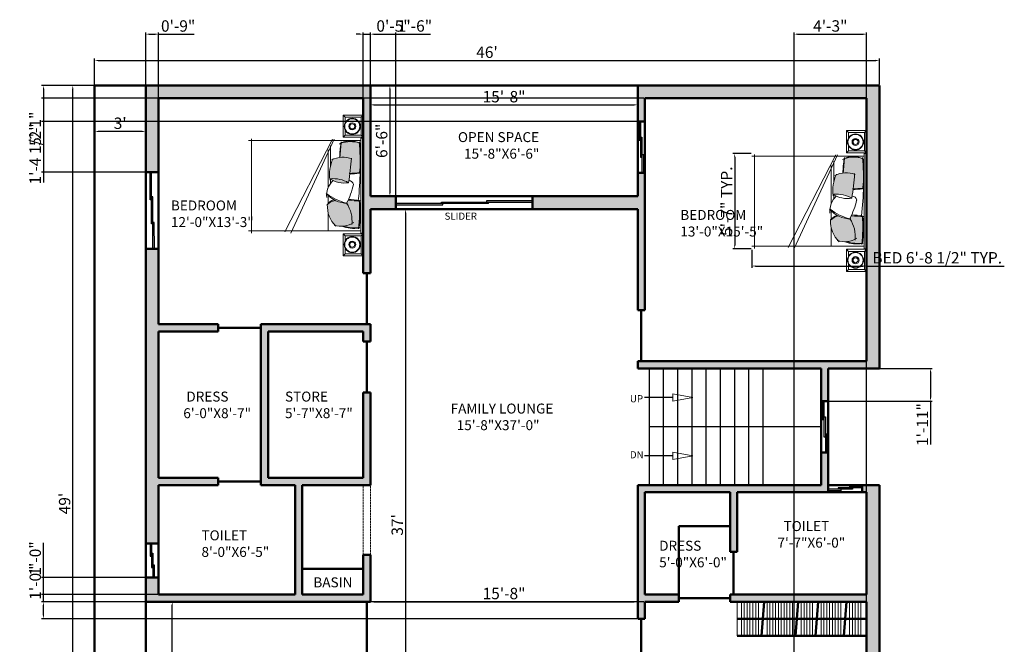
# Model space of a CAD drawing. Units: inches. Extents: x 1913 to 5309, y 1003 to 1733.
# Tile 23 of 23: x 4616 to 5309, y 1294 to 1733. Entities that reach past the tile are written whole.
import ezdxf

# ---------------------------------------------------------------- set-up
doc = ezdxf.new("R2010")
doc.units = ezdxf.units.IN
doc.linetypes.add('HIDDEN2', pattern=[0.1875, 0.125, -0.0625])
for name, color, linetype, lineweight in [('0.10', 252, 'Continuous', 9), ('0.15', 34, 'Continuous', 15), ('A-ANNO-DIMS', 2, 'Continuous', 18), ('A-ANNO-SYMB', 1, 'Continuous', 18), ('A-ANNO-TEXT', 7, 'Continuous', 18), ('A-AREA-IDEN', 3, 'Continuous', 18), ('A-FLOR-PATT', 252, 'Continuous', 13), ('A-FLOR-STRS', 7, 'Continuous', 25), ('A-FURN', 8, 'Continuous', 18), ('A-FURN-PATT', 8, 'Continuous', 13), ('A-GLAZ', 5, 'Continuous', 25), ('A-WALL', 7, 'Continuous', 50), ('A-WALL-OVHD', 8, 'HIDDEN2', 18)]:
    doc.layers.add(name, color=color, linetype=linetype, lineweight=lineweight)
doc.styles.get("Standard").update_dxf_attribs({"font": 'arial.ttf'})
doc.dimstyles.new('ISO-25', dxfattribs={"dimtxt": 8, "dimasz": 2.5, "dimexe": 1.25, "dimexo": 0.625, "dimtad": 1, "dimdec": 1, "dimlunit": 3, "dimtxsty": 'Standard', "dimcen": 2.5, "dimclrd": 256, "dimclrt": 1, "dimadec": 0, "dimazin": 0, "dimtfac": 1, "dimtdec": 1, "dimtmove": 0, "dimatfit": 3, "dimfxl": 1, "dimarcsym": 0})

# ---------------------------------------------------------------- blocks, each defined once
blk = doc.blocks.new('camita')
at = {"layer": '0.10'}
for p, q in [((-0.85, -0.045), (0.85, -0.045)), ((-0.805, -0.045), (-0.805, -2.048)), ((0.805, -0.045), (0.805, -2.048)), ((-0.827, -0.521), (0.846, -1.293)), ((-0.827, -0.548), (0.824, -1.399)), ((-0.716, -0.585), (-0.355, -0.585)), ((-0.638, -0.63), (0.043, -0.63)), ((-0.114, -0.585), (-0.049, -0.585)), ((0.175, -0.63), (0.318, -0.63)), ((0.474, -0.63), (0.805, -0.63)), ((-0.835, -2), (0.846, -2))]:
    blk.add_line(p, q, dxfattribs=at)
blk.add_lwpolyline([(-0.85, -0.041), (0.85, -0.041), (0.85, 0), (-0.85, 0)], close=True, dxfattribs=at)
for centre, radius, start, end in [((-0.457, -0.236), 0.344, 147.51, 213.8336), ((-0.2, -0.227), 0.586, 163.9263, 197.1409), ((-0.364, -5.846), 5.791, 83.8073, 94.1211), ((-0.51, -1.723), 1.678, 80.1255, 98.6619), ((2.353, -0.053), 2.58, 180.1063, 184.3854), ((-1.544, -0.245), 1.333, 359.9394, 7.5533), ((1.581, -0.289), 1.335, 170.3802, 178.9914), ((-1.44, -0.061), 1.712, 352.9291, 0.3959), ((0.452, -3.067), 3, 83.9026, 93.6759), ((0.486, -1.629), 1.578, 80.1602, 98.06), ((0.32, -0.394), 0.404, 341.4524, 33.4512), ((0.029, -0.138), 0.726, 342.5841, 6.0048), ((0.133, -0.17), 0.631, 339.923, 8.7433), ((-0.054, -0.363), 0.454, 159.3026, 206.5026), ((-1.33, -9.675), 9.499, 82.2708, 84.9399), ((0.458, -0.545), 0.584, 151.0456, 184.1497), ((-0.534, -0.339), 0.487, 327.2644, 9.0473), ((-0.007, -0.258), 0.0828, 100.018, 179.736), ((-0.293, -1.438), 1.29, 61.9749, 77.8435), ((-0.199, -0.274), 0.516, 310.7395, 359.0576), ((-0.567, -0.087), 0.906, 321.6953, 346.4626), ((0.627, -0.752), 0.551, 82.9691, 124.6739), ((-1.867, -14.986), 14.632, 84.6597, 85.7516), ((-0.46, 1.486), 1.909, 260.953, 268.6517), ((0.571, -0.432), 0.315, 192.9388, 221.9636), ((0.361, -0.133), 0.51, 267.2589, 315.2997), ((-0.2, 0.064), 0.667, 244.7809, 279.0606), ((0.179, -0.272), 0.383, 224.5284, 275.2229), ((0.438, -0.483), 0.19, 193.6849, 236.7035)]:
    blk.add_arc(centre, radius, start, end, dxfattribs=at)
blk = doc.blocks.new('VELADOR')
at = {"layer": '0.15'}
for p, q in [((-0.248, 0), (-0.203, -0.045)), ((0.248, 0), (0.202, -0.045)), ((-0.203, -0.405), (-0.248, -0.45)), ((0.248, -0.45), (0.202, -0.405))]:
    blk.add_line(p, q, dxfattribs=at)
blk.add_lwpolyline([(-0.248, 0), (-0.248, -0.45), (0.248, -0.45), (0.248, 0)], close=True, dxfattribs=at)
blk.add_lwpolyline([(0.092, -0.405), (0.202, -0.405), (0.202, -0.045), (-0.203, -0.045), (-0.203, -0.405), (-0.082, -0.405)], dxfattribs=at)
for radius in [0.18, 0.169, 0.0788, 0.0563]:
    blk.add_circle((0.005, -0.247), radius, dxfattribs=at)
blk = doc.blocks.new('*D29')
at = {"layer": 'A-ANNO-DIMS', "color": 0, "lineweight": -2, "transparency": 16777216}
for p, q in [((4668.01, 1686.96), (4652.03, 1686.96)), ((4653.28, 1101.46), (4653.28, 1684.46)), ((4668.01, 1098.96), (4652.03, 1098.96))]:
    blk.add_line(p, q, dxfattribs=at)
at = {"layer": 'A-ANNO-DIMS', "color": 0, "transparency": 16777216}
for points in [[(4652.86, 1684.46), (4653.69, 1684.46), (4653.28, 1686.96)], [(4652.86, 1101.46), (4653.69, 1101.46), (4653.28, 1098.96)]]:
    blk.add_solid(points, dxfattribs=at)
at = {"layer": 'Defpoints', "color": 0, "transparency": 16777216}
for p in [(4653.28, 1686.96), (4668.63, 1686.96), (4668.63, 1098.96)]:
    blk.add_point(p, dxfattribs=at)
at = {"layer": 'A-ANNO-DIMS', "color": 0, "transparency": 16777216, "insert": (4648.57, 1392.96), "char_height": 8, "attachment_point": 5, "rotation": 90}
blk.add_mtext("49'", dxfattribs=at)
blk = doc.blocks.new('*D30')
at = {"layer": 'A-ANNO-DIMS', "color": 0, "lineweight": -2, "transparency": 16777216}
for p, q in [((4668.63, 1687.59), (4668.63, 1705.75)), ((4671.13, 1704.5), (5218.13, 1704.5)), ((5220.63, 1687.59), (5220.63, 1705.75))]:
    blk.add_line(p, q, dxfattribs=at)
at = {"layer": 'A-ANNO-DIMS', "color": 0, "transparency": 16777216}
for points in [[(4671.13, 1704.92), (4671.13, 1704.08), (4668.63, 1704.5)], [(5218.13, 1704.92), (5218.13, 1704.08), (5220.63, 1704.5)]]:
    blk.add_solid(points, dxfattribs=at)
at = {"layer": 'Defpoints', "color": 0, "transparency": 16777216}
for p in [(5220.63, 1704.5), (4668.63, 1686.96), (5220.63, 1686.96)]:
    blk.add_point(p, dxfattribs=at)
at = {"layer": 'A-ANNO-DIMS', "color": 0, "transparency": 16777216, "insert": (4944.63, 1709.21), "char_height": 8, "attachment_point": 5}
blk.add_mtext("46'", dxfattribs=at)
blk = doc.blocks.new('*D31')
at = {"layer": 'A-ANNO-DIMS', "color": 0, "lineweight": -2, "transparency": 16777216}
for p, q in [((4862.63, 1679.78), (4862.63, 1672.02)), ((5050.63, 1679.78), (5050.63, 1672.02)), ((4865.13, 1673.27), (5048.13, 1673.27))]:
    blk.add_line(p, q, dxfattribs=at)
at = {"layer": 'A-ANNO-DIMS', "color": 0, "transparency": 16777216}
for points in [[(4865.13, 1673.68), (4865.13, 1672.85), (4862.63, 1673.27)], [(5048.13, 1673.68), (5048.13, 1672.85), (5050.63, 1673.27)]]:
    blk.add_solid(points, dxfattribs=at)
at = {"layer": 'Defpoints', "color": 0, "transparency": 16777216}
for p in [(4862.63, 1680.41), (5050.63, 1680.41), (5050.63, 1673.27)]:
    blk.add_point(p, dxfattribs=at)
at = {"layer": 'A-ANNO-DIMS', "color": 0, "transparency": 16777216, "insert": (4956.63, 1677.98), "char_height": 8, "attachment_point": 5}
blk.add_mtext('15\'-8"', dxfattribs=at)
blk = doc.blocks.new('*D32')
at = {"layer": 'A-ANNO-DIMS', "color": 0, "lineweight": -2, "transparency": 16777216}
for p, q in [((4876.45, 1686.96), (4875.07, 1686.96)), ((4876.32, 1684.46), (4876.32, 1611.46)), ((4876.45, 1608.96), (4875.07, 1608.96))]:
    blk.add_line(p, q, dxfattribs=at)
at = {"layer": 'A-ANNO-DIMS', "color": 0, "transparency": 16777216}
for points in [[(4875.91, 1684.46), (4876.74, 1684.46), (4876.32, 1686.96)], [(4875.91, 1611.46), (4876.74, 1611.46), (4876.32, 1608.96)]]:
    blk.add_solid(points, dxfattribs=at)
at = {"layer": 'Defpoints', "color": 0, "transparency": 16777216}
for p in [(4877.08, 1686.96), (4876.32, 1608.96), (4877.08, 1608.96)]:
    blk.add_point(p, dxfattribs=at)
at = {"layer": 'A-ANNO-DIMS', "color": 0, "transparency": 16777216, "insert": (4871.61, 1647.96), "char_height": 8, "attachment_point": 5, "rotation": 90}
blk.add_mtext('6\'-6"', dxfattribs=at)
blk = doc.blocks.new('*D33')
at = {"layer": 'A-ANNO-DIMS', "color": 0, "lineweight": -2, "transparency": 16777216}
for p, q in [((4722.69, 1323.96), (4724.5, 1323.96)), ((4723.25, 1149.46), (4723.25, 1321.46)), ((4722.69, 1146.96), (4724.5, 1146.96))]:
    blk.add_line(p, q, dxfattribs=at)
at = {"layer": 'A-ANNO-DIMS', "color": 0, "transparency": 16777216}
for points in [[(4722.83, 1321.46), (4723.66, 1321.46), (4723.25, 1323.96)], [(4722.83, 1149.46), (4723.66, 1149.46), (4723.25, 1146.96)]]:
    blk.add_solid(points, dxfattribs=at)
at = {"layer": 'Defpoints', "color": 0, "transparency": 16777216}
for p in [(4722.06, 1323.96), (4723.25, 1323.96), (4722.06, 1146.96)]:
    blk.add_point(p, dxfattribs=at)
at = {"layer": 'A-ANNO-DIMS', "color": 0, "transparency": 16777216, "insert": (4718.54, 1235.46), "char_height": 8, "attachment_point": 5, "rotation": 90}
blk.add_mtext('14\'-9"', dxfattribs=at)
blk = doc.blocks.new('*D35')
at = {"layer": 'A-ANNO-DIMS', "color": 0, "lineweight": -2, "transparency": 16777216}
for p, q in [((4668.63, 1655.19), (4668.63, 1655.82)), ((4704.63, 1655.19), (4704.63, 1655.82)), ((4702.13, 1654.57), (4671.13, 1654.57))]:
    blk.add_line(p, q, dxfattribs=at)
at = {"layer": 'A-ANNO-DIMS', "color": 0, "transparency": 16777216}
for points in [[(4671.13, 1654.99), (4671.13, 1654.15), (4668.63, 1654.57)], [(4702.13, 1654.99), (4702.13, 1654.15), (4704.63, 1654.57)]]:
    blk.add_solid(points, dxfattribs=at)
at = {"layer": 'Defpoints', "color": 0, "transparency": 16777216}
for p in [(4668.63, 1654.57), (4668.63, 1654.57), (4704.63, 1654.57)]:
    blk.add_point(p, dxfattribs=at)
at = {"layer": 'A-ANNO-DIMS', "color": 0, "transparency": 16777216, "insert": (4686.63, 1659.28), "char_height": 8, "attachment_point": 5}
blk.add_mtext("3'", dxfattribs=at)
blk = doc.blocks.new('*D39')
at = {"layer": 'A-ANNO-DIMS', "color": 0, "lineweight": -2, "transparency": 16777216}
for p, q in [((4881.23, 1599.96), (4888.52, 1599.96)), ((4887.27, 1597.46), (4887.27, 1158.43)), ((4881.23, 1155.93), (4888.52, 1155.93))]:
    blk.add_line(p, q, dxfattribs=at)
at = {"layer": 'A-ANNO-DIMS', "color": 0, "transparency": 16777216}
for points in [[(4886.85, 1597.46), (4887.69, 1597.46), (4887.27, 1599.96)], [(4886.85, 1158.43), (4887.69, 1158.43), (4887.27, 1155.93)]]:
    blk.add_solid(points, dxfattribs=at)
at = {"layer": 'Defpoints', "color": 0, "transparency": 16777216}
for p in [(4880.6, 1599.96), (4880.6, 1155.93), (4887.27, 1155.93)]:
    blk.add_point(p, dxfattribs=at)
at = {"layer": 'A-ANNO-DIMS', "color": 0, "transparency": 16777216, "insert": (4882.56, 1377.95), "char_height": 8, "attachment_point": 5, "rotation": 90}
blk.add_mtext("37'", dxfattribs=at)
blk = doc.blocks.new('*D40')
at = {"layer": 'A-ANNO-DIMS', "color": 0, "lineweight": -2, "transparency": 16777216}
for p, q in [((4862.63, 1324.59), (4862.63, 1325.21)), ((4865.13, 1323.96), (5048.13, 1323.96)), ((5050.63, 1324.59), (5050.63, 1325.21))]:
    blk.add_line(p, q, dxfattribs=at)
at = {"layer": 'A-ANNO-DIMS', "color": 0, "transparency": 16777216}
for points in [[(4865.13, 1324.38), (4865.13, 1323.55), (4862.63, 1323.96)], [(5048.13, 1324.38), (5048.13, 1323.55), (5050.63, 1323.96)]]:
    blk.add_solid(points, dxfattribs=at)
at = {"layer": 'Defpoints', "color": 0, "transparency": 16777216}
for p in [(4862.63, 1323.96), (5050.63, 1323.96), (5050.63, 1323.96)]:
    blk.add_point(p, dxfattribs=at)
at = {"layer": 'A-ANNO-DIMS', "color": 0, "transparency": 16777216, "insert": (4956.63, 1328.67), "char_height": 8, "attachment_point": 5}
blk.add_mtext('15\'-8"', dxfattribs=at)
blk = doc.blocks.new('WIN-24')
for p, q in [((0, 15), (0, 24)), ((1, 7), (1, 24)), ((1, 15), (0, 15)), ((2, 17), (1, 17)), ((2, 0), (2, 17)), ((2, 7), (1, 7)), ((3, 9), (2, 9)), ((3, 0), (3, 9))]:
    blk.add_line(p, q)
blk = doc.blocks.new('WIN-54')
for p, q in [((0, 54), (0, 35)), ((1, 54), (1, 17)), ((0, 35), (1, 35)), ((1, 36), (2, 36)), ((2, 36), (2, 0)), ((1, 17), (2, 17)), ((2, 19), (3, 19)), ((3, 19), (3, 0))]:
    blk.add_line(p, q)
blk = doc.blocks.new('WIN-36')
for p, q in [((0, 23), (0, 36)), ((1, 11), (1, 36)), ((1, 23), (0, 23)), ((2, 25), (1, 25)), ((2, 0), (2, 25)), ((2, 11), (1, 11)), ((3, 13), (2, 13)), ((3, 0), (3, 13))]:
    blk.add_line(p, q)
blk = doc.blocks.new('WIN-SLIDER-96')
for p, q in [((65, 1), (0, 1)), ((0, 0), (33, 0)), ((32, 2), (96, 2)), ((32, 1), (32, 2)), ((33, 0), (33, 1)), ((64, 3), (96, 3)), ((64, 2), (64, 3)), ((65, 1), (65, 2))]:
    blk.add_line(p, q)
blk = doc.blocks.new('*D61')
at = {"layer": 'A-ANNO-DIMS', "color": 0, "lineweight": -2, "transparency": 16777216}
for p, q in [((5130.98, 1571.43), (5130.98, 1558.7)), ((5211.63, 1571.43), (5211.63, 1558.7))]:
    blk.add_line(p, q, dxfattribs=at)
at = {"layer": 'A-ANNO-DIMS', "lineweight": -2, "transparency": 16777216}
for p, q in [((5133.48, 1559.95), (5209.13, 1559.95)), ((5211.63, 1559.95), (5308.52, 1559.95))]:
    blk.add_line(p, q, dxfattribs=at)
at = {"layer": 'A-ANNO-DIMS', "transparency": 16777216}
for points in [[(5133.48, 1560.37), (5133.48, 1559.54), (5130.98, 1559.95)], [(5209.13, 1560.37), (5209.13, 1559.54), (5211.63, 1559.95)]]:
    blk.add_solid(points, dxfattribs=at)
at = {"layer": 'Defpoints', "color": 0, "transparency": 16777216}
for p in [(5130.98, 1572.05), (5211.63, 1572.05), (5211.63, 1559.95)]:
    blk.add_point(p, dxfattribs=at)
at = {"layer": 'A-ANNO-DIMS', "color": 1, "transparency": 16777216, "insert": (5261.33, 1564.71), "char_height": 8, "attachment_point": 5}
blk.add_mtext('BED 6\'-8 1/2" TYP.', dxfattribs=at)
blk = doc.blocks.new('*D62')
at = {"layer": 'A-ANNO-DIMS', "color": 0, "lineweight": -2, "transparency": 16777216}
for p, q in [((5130.35, 1638.99), (5117.63, 1638.99)), ((5130.35, 1572.05), (5117.63, 1572.05))]:
    blk.add_line(p, q, dxfattribs=at)
at = {"layer": 'A-ANNO-DIMS', "lineweight": -2, "transparency": 16777216}
blk.add_line((5118.88, 1636.49), (5118.88, 1574.55), dxfattribs=at)
at = {"layer": 'A-ANNO-DIMS', "transparency": 16777216}
for points in [[(5118.46, 1636.49), (5119.29, 1636.49), (5118.88, 1638.99)], [(5118.46, 1574.55), (5119.29, 1574.55), (5118.88, 1572.05)]]:
    blk.add_solid(points, dxfattribs=at)
at = {"layer": 'Defpoints', "color": 0, "transparency": 16777216}
for p in [(5130.98, 1638.99), (5118.88, 1572.05), (5130.98, 1572.05)]:
    blk.add_point(p, dxfattribs=at)
at = {"layer": 'A-ANNO-DIMS', "color": 1, "transparency": 16777216, "insert": (5114.18, 1605.52), "char_height": 8, "attachment_point": 5, "rotation": 90}
blk.add_mtext('5\'-7" TYP.', dxfattribs=at)
blk = doc.blocks.new('*D128')
at = {"layer": 'A-ANNO-DIMS', "color": 0, "lineweight": -2, "transparency": 16777216}
for p, q in [((4704.63, 1687.59), (4704.63, 1724.21)), ((4713.63, 1678.59), (4713.63, 1724.21))]:
    blk.add_line(p, q, dxfattribs=at)
at = {"layer": 'A-ANNO-DIMS', "lineweight": -2, "transparency": 16777216}
for p, q in [((4707.13, 1722.96), (4711.13, 1722.96)), ((4713.63, 1722.96), (4738.65, 1722.96))]:
    blk.add_line(p, q, dxfattribs=at)
at = {"layer": 'A-ANNO-DIMS', "transparency": 16777216}
for points in [[(4707.13, 1723.38), (4707.13, 1722.55), (4704.63, 1722.96)], [(4711.13, 1723.38), (4711.13, 1722.55), (4713.63, 1722.96)]]:
    blk.add_solid(points, dxfattribs=at)
at = {"layer": 'Defpoints', "color": 0, "transparency": 16777216}
for p in [(4713.63, 1722.96), (4704.63, 1686.96), (4713.63, 1677.96)]:
    blk.add_point(p, dxfattribs=at)
at = {"layer": 'A-ANNO-DIMS', "color": 1, "transparency": 16777216, "insert": (4727.39, 1727.67), "char_height": 8, "attachment_point": 5}
blk.add_mtext('0\'-9"', dxfattribs=at)
blk = doc.blocks.new('*D129')
at = {"layer": 'A-ANNO-DIMS', "lineweight": -2, "transparency": 16777216}
for p, q in [((4855.13, 1722.96), (4852.63, 1722.96)), ((4857.63, 1722.96), (4862.63, 1722.96)), ((4865.13, 1722.96), (4890.15, 1722.96))]:
    blk.add_line(p, q, dxfattribs=at)
at = {"layer": 'A-ANNO-DIMS', "color": 0, "lineweight": -2, "transparency": 16777216}
for p, q in [((4857.63, 1678.59), (4857.63, 1724.21)), ((4862.63, 1687.59), (4862.63, 1724.21))]:
    blk.add_line(p, q, dxfattribs=at)
at = {"layer": 'A-ANNO-DIMS', "transparency": 16777216}
for points in [[(4855.13, 1723.38), (4855.13, 1722.55), (4857.63, 1722.96)], [(4865.13, 1723.38), (4865.13, 1722.55), (4862.63, 1722.96)]]:
    blk.add_solid(points, dxfattribs=at)
at = {"layer": 'Defpoints', "color": 0, "transparency": 16777216}
for p in [(4862.63, 1722.96), (4862.63, 1686.96), (4857.63, 1677.96)]:
    blk.add_point(p, dxfattribs=at)
at = {"layer": 'A-ANNO-DIMS', "color": 1, "transparency": 16777216, "insert": (4878.89, 1727.67), "char_height": 8, "attachment_point": 5}
blk.add_mtext('0\'-5"', dxfattribs=at)
blk = doc.blocks.new('*D130')
at = {"layer": 'A-ANNO-DIMS', "color": 0, "lineweight": -2, "transparency": 16777216}
for p, q in [((4704.01, 1686.96), (4631.38, 1686.96)), ((4704.01, 1625.96), (4631.38, 1625.96))]:
    blk.add_line(p, q, dxfattribs=at)
at = {"layer": 'A-ANNO-DIMS', "lineweight": -2, "transparency": 16777216}
blk.add_line((4632.63, 1684.46), (4632.63, 1628.46), dxfattribs=at)
at = {"layer": 'A-ANNO-DIMS', "transparency": 16777216}
for points in [[(4632.22, 1684.46), (4633.05, 1684.46), (4632.63, 1686.96)], [(4632.22, 1628.46), (4633.05, 1628.46), (4632.63, 1625.96)]]:
    blk.add_solid(points, dxfattribs=at)
at = {"layer": 'Defpoints', "color": 0, "transparency": 16777216}
for p in [(4704.63, 1686.96), (4632.63, 1625.96), (4704.63, 1625.96)]:
    blk.add_point(p, dxfattribs=at)
at = {"layer": 'A-ANNO-DIMS', "color": 1, "transparency": 16777216, "insert": (4627.92, 1656.46), "char_height": 8, "attachment_point": 5, "rotation": 90}
blk.add_mtext('5\'-1"', dxfattribs=at)
blk = doc.blocks.new('*D131')
at = {"layer": 'A-ANNO-DIMS', "lineweight": -2, "transparency": 16777216}
for p, q in [((4632.63, 1340.96), (4632.63, 1365.23)), ((4632.63, 1331.46), (4632.63, 1338.46))]:
    blk.add_line(p, q, dxfattribs=at)
at = {"layer": 'A-ANNO-DIMS', "color": 0, "lineweight": -2, "transparency": 16777216}
for p, q in [((4713.01, 1340.96), (4631.38, 1340.96)), ((4713.01, 1328.96), (4631.38, 1328.96))]:
    blk.add_line(p, q, dxfattribs=at)
at = {"layer": 'A-ANNO-DIMS', "transparency": 16777216}
for points in [[(4632.22, 1338.46), (4633.05, 1338.46), (4632.63, 1340.96)], [(4632.22, 1331.46), (4633.05, 1331.46), (4632.63, 1328.96)]]:
    blk.add_solid(points, dxfattribs=at)
at = {"layer": 'Defpoints', "color": 0, "transparency": 16777216}
for p in [(4632.63, 1340.96), (4713.63, 1340.96), (4713.63, 1328.96)]:
    blk.add_point(p, dxfattribs=at)
at = {"layer": 'A-ANNO-DIMS', "color": 1, "transparency": 16777216, "insert": (4627.92, 1354.35), "char_height": 8, "attachment_point": 5, "rotation": 90}
blk.add_mtext('1\'-0"', dxfattribs=at)
blk = doc.blocks.new('*D132')
at = {"layer": 'A-ANNO-DIMS', "color": 0, "lineweight": -2, "transparency": 16777216}
for p, q in [((5055.01, 1677.96), (4631.38, 1677.96)), ((5055.01, 1661.46), (4631.38, 1661.46))]:
    blk.add_line(p, q, dxfattribs=at)
at = {"layer": 'A-ANNO-DIMS', "lineweight": -2, "transparency": 16777216}
for p, q in [((4632.63, 1675.46), (4632.63, 1663.96)), ((4632.63, 1661.46), (4632.63, 1618.56))]:
    blk.add_line(p, q, dxfattribs=at)
at = {"layer": 'A-ANNO-DIMS', "transparency": 16777216}
for points in [[(4632.22, 1675.46), (4633.05, 1675.46), (4632.63, 1677.96)], [(4632.22, 1663.96), (4633.05, 1663.96), (4632.63, 1661.46)]]:
    blk.add_solid(points, dxfattribs=at)
at = {"layer": 'Defpoints', "color": 0, "transparency": 16777216}
for p in [(5055.63, 1677.96), (4632.63, 1661.46), (5055.63, 1661.46)]:
    blk.add_point(p, dxfattribs=at)
at = {"layer": 'A-ANNO-DIMS', "color": 1, "transparency": 16777216, "insert": (4627.87, 1638.76), "char_height": 8, "attachment_point": 5, "rotation": 90}
blk.add_mtext('1\'-4 1/2"', dxfattribs=at)
blk = doc.blocks.new('*D133')
at = {"layer": 'A-ANNO-DIMS', "color": 0, "lineweight": -2, "transparency": 16777216}
for p, q in [((4862.63, 1609.59), (4862.63, 1724.21)), ((4880.6, 1609.59), (4880.6, 1724.21))]:
    blk.add_line(p, q, dxfattribs=at)
at = {"layer": 'A-ANNO-DIMS', "lineweight": -2, "transparency": 16777216}
for p, q in [((4865.13, 1722.96), (4878.1, 1722.96)), ((4880.6, 1722.96), (4904.87, 1722.96))]:
    blk.add_line(p, q, dxfattribs=at)
at = {"layer": 'A-ANNO-DIMS', "transparency": 16777216}
for points in [[(4865.13, 1723.38), (4865.13, 1722.55), (4862.63, 1722.96)], [(4878.1, 1723.38), (4878.1, 1722.55), (4880.6, 1722.96)]]:
    blk.add_solid(points, dxfattribs=at)
at = {"layer": 'Defpoints', "color": 0, "transparency": 16777216}
for p in [(4880.6, 1722.96), (4862.63, 1608.96), (4880.6, 1608.96)]:
    blk.add_point(p, dxfattribs=at)
at = {"layer": 'A-ANNO-DIMS', "color": 1, "transparency": 16777216, "insert": (4893.98, 1727.67), "char_height": 8, "attachment_point": 5}
blk.add_mtext('1\'-6"', dxfattribs=at)
blk = doc.blocks.new('*D134')
at = {"layer": 'A-ANNO-DIMS', "color": 0, "lineweight": -2, "transparency": 16777216}
for p, q in [((5185.26, 1487.96), (5257.88, 1487.96)), ((5185.26, 1464.96), (5257.88, 1464.96))]:
    blk.add_line(p, q, dxfattribs=at)
at = {"layer": 'A-ANNO-DIMS', "lineweight": -2, "transparency": 16777216}
for p, q in [((5256.63, 1485.46), (5256.63, 1467.46)), ((5256.63, 1464.96), (5256.63, 1434.49))]:
    blk.add_line(p, q, dxfattribs=at)
at = {"layer": 'A-ANNO-DIMS', "transparency": 16777216}
for points in [[(5256.22, 1485.46), (5257.05, 1485.46), (5256.63, 1487.96)], [(5256.22, 1467.46), (5257.05, 1467.46), (5256.63, 1464.96)]]:
    blk.add_solid(points, dxfattribs=at)
at = {"layer": 'Defpoints', "color": 0, "transparency": 16777216}
for p in [(5184.63, 1487.96), (5184.63, 1464.96), (5256.63, 1464.96)]:
    blk.add_point(p, dxfattribs=at)
at = {"layer": 'A-ANNO-DIMS', "color": 1, "transparency": 16777216, "insert": (5251.99, 1448.47), "char_height": 8, "attachment_point": 5, "rotation": 90}
blk.add_mtext('1\'-11"', dxfattribs=at)
blk = doc.blocks.new('*D138')
at = {"layer": 'A-ANNO-DIMS', "color": 0, "lineweight": -2, "transparency": 16777216}
for p, q in [((5160.63, 1180.59), (5160.63, 1724.21)), ((5211.63, 1180.59), (5211.63, 1724.21))]:
    blk.add_line(p, q, dxfattribs=at)
at = {"layer": 'A-ANNO-DIMS', "lineweight": -2, "transparency": 16777216}
blk.add_line((5163.13, 1722.96), (5209.13, 1722.96), dxfattribs=at)
at = {"layer": 'A-ANNO-DIMS', "transparency": 16777216}
for points in [[(5163.13, 1723.38), (5163.13, 1722.55), (5160.63, 1722.96)], [(5209.13, 1723.38), (5209.13, 1722.55), (5211.63, 1722.96)]]:
    blk.add_solid(points, dxfattribs=at)
at = {"layer": 'Defpoints', "color": 0, "transparency": 16777216}
for p in [(5211.63, 1722.96), (5160.63, 1179.96), (5211.63, 1179.96)]:
    blk.add_point(p, dxfattribs=at)
at = {"layer": 'A-ANNO-DIMS', "color": 1, "transparency": 16777216, "insert": (5186.13, 1727.68), "char_height": 8, "attachment_point": 5}
blk.add_mtext('4\'-3"', dxfattribs=at)
blk = doc.blocks.new('*D139')
at = {"layer": 'A-ANNO-DIMS', "lineweight": -2, "transparency": 16777216}
for p, q in [((4632.63, 1323.96), (4632.63, 1348.23)), ((4632.63, 1314.46), (4632.63, 1321.46))]:
    blk.add_line(p, q, dxfattribs=at)
at = {"layer": 'A-ANNO-DIMS', "color": 0, "lineweight": -2, "transparency": 16777216}
for p, q in [((5055.01, 1323.96), (4631.38, 1323.96)), ((5050.01, 1311.96), (4631.38, 1311.96))]:
    blk.add_line(p, q, dxfattribs=at)
at = {"layer": 'A-ANNO-DIMS', "transparency": 16777216}
for points in [[(4632.22, 1321.46), (4633.05, 1321.46), (4632.63, 1323.96)], [(4632.22, 1314.46), (4633.05, 1314.46), (4632.63, 1311.96)]]:
    blk.add_solid(points, dxfattribs=at)
at = {"layer": 'Defpoints', "color": 0, "transparency": 16777216}
for p in [(4632.63, 1323.96), (5055.63, 1323.96), (5050.63, 1311.96)]:
    blk.add_point(p, dxfattribs=at)
at = {"layer": 'A-ANNO-DIMS', "color": 1, "transparency": 16777216, "insert": (4627.92, 1337.35), "char_height": 8, "attachment_point": 5, "rotation": 90}
blk.add_mtext('1\'-0"', dxfattribs=at)

msp = doc.modelspace()

# ---------------------------------------------------------------- hatches: boundary and pattern name
at = {"layer": 'A-FLOR-PATT'}
h = msp.add_hatch(color=256, dxfattribs=at)
h.dxf.hatch_style = 1
h.paths.add_polyline_path([(4862.63, 1686.96), (4704.63, 1686.96), (4704.63, 1625.96), (4713.63, 1625.96), (4713.63, 1677.96), (4857.63, 1677.96), (4857.63, 1554.96), (4862.63, 1554.96), (4862.63, 1599.96), (4880.6, 1599.96), (4880.6, 1608.96), (4862.63, 1608.96)])
h.paths.add_polyline_path([(5055.63, 1625.46), (5050.63, 1625.46), (5050.63, 1608.96), (4976.6, 1608.96), (4976.6, 1599.96), (5050.63, 1599.96), (5050.63, 1528.96), (5055.63, 1528.96)])
h.paths.add_polyline_path([(5220.63, 1686.96), (5050.63, 1686.96), (5050.63, 1661.46), (5055.63, 1661.46), (5055.63, 1677.96), (5211.63, 1677.96), (5211.63, 1492.96), (5050.63, 1492.96), (5050.63, 1487.96), (5179.63, 1487.96), (5179.63, 1464.96), (5184.63, 1464.96), (5184.63, 1487.96), (5220.63, 1487.96)])
h.paths.add_polyline_path([(5120.63, 1400.96), (5184.63, 1400.96), (5184.63, 1428.96), (5179.63, 1428.96), (5179.63, 1405.96), (5050.63, 1405.96), (5050.63, 1311.96), (5055.63, 1311.96), (5055.63, 1323.96), (5079.63, 1323.96), (5079.63, 1328.96), (5055.63, 1328.96), (5055.63, 1400.96), (5115.63, 1400.96), (5115.63, 1358.96), (5120.63, 1358.96)])
h.paths.add_polyline_path([(5220.63, 1405.96), (5208.63, 1405.96), (5208.63, 1400.96), (5211.63, 1400.96), (5211.63, 1328.96), (5115.63, 1328.96), (5115.63, 1323.96), (5211.63, 1323.96), (5211.63, 1299.96), (5211.63, 1179.96), (5197.5, 1179.96), (5160.63, 1179.96), (5160.63, 1170.96), (5211.63, 1170.96), (5211.63, 1146.96), (5220.63, 1146.96)])
h.paths.add_polyline_path([(5106.63, 1179.96), (5085.63, 1179.96), (5085.63, 1170.96), (5106.63, 1170.96)])
h.paths.add_polyline_path([(5050.63, 1158.98), (5050.63, 1199.59, 0.414216), (5047.62, 1202.59), (5031.77, 1202.59, 0.414214), (5028.76, 1199.59), (5028.76, 1181.52, 0.46174), (5030.5, 1180.04), (5047.41, 1180.04, 0.414263), (5046.81, 1179.45), (5046.81, 1162.57, 0.41435), (5047.41, 1161.97), (5028.67, 1161.97, 0.41842), (5028.08, 1161.36, 0.785879), (5027.16, 1162.09, 0.298637), (5028.06, 1163.46), (5028.06, 1178.53, 0.414214), (5026.56, 1180.02), (5011.51, 1180.02, 0.416116), (5010.01, 1178.51, 0.414208), (5008.5, 1180.02), (5008.5, 1180.02, -0.413869), (5009.99, 1178.52, -0.412492), (5011.5, 1180.02), (5011.5, 1180.03), (5026.56, 1180.02, -0.414213), (5028.06, 1178.53, -0.414214), (5029.56, 1180.02), (5029.44, 1180.27, -0.252555), (5028.76, 1181.52), (5028.74, 1181.51), (5028.76, 1199.59, -0.414214), (5031.77, 1202.59), (5047.63, 1202.59, -0.414214), (5050.63, 1199.59), (5050.63, 1275.96), (5055.63, 1275.96), (5055.63, 1146.96), (5032.63, 1146.96), (5032.63, 1155.96), (4972.36, 1155.96, -0.414214), (4969.35, 1158.97), (4969.35, 1158.97, 0.421637), (4972.44, 1155.96), (5047.7, 1155.96, 0.407251)])
h.paths.add_polyline_path([(4866.63, 1275.96), (4857.63, 1275.96), (4857.63, 1233.96), (4866.63, 1233.96), (4866.63, 1237.71)])
h.paths.add_polyline_path([(4866.63, 1173.96), (4857.63, 1173.96), (4857.63, 1146.96), (4884.63, 1146.96), (4884.63, 1155.93), (4869.77, 1155.93, -0.414214), (4866.63, 1159.07)])
h.paths.add_polyline_path([(4862.63, 1356.96), (4857.63, 1356.96), (4857.63, 1328.96), (4814.63, 1328.96), (4814.63, 1405.96), (4862.63, 1405.96), (4862.63, 1470.96), (4857.63, 1470.96), (4857.63, 1410.96), (4790.63, 1410.96), (4790.63, 1513.96), (4857.63, 1513.96), (4857.63, 1506.96), (4862.63, 1506.96), (4862.63, 1518.96), (4785.63, 1518.96), (4785.63, 1405.96), (4809.63, 1405.96), (4809.63, 1328.96), (4713.63, 1328.96), (4713.63, 1340.96), (4704.63, 1340.96), (4704.63, 1323.96), (4862.63, 1323.96)])
h.paths.add_polyline_path([(4713.63, 1513.96), (4755.63, 1513.96), (4755.63, 1518.96), (4713.63, 1518.96), (4713.63, 1571.96), (4704.63, 1571.96), (4704.63, 1420.96), (4704.63, 1364.96), (4713.63, 1364.96), (4713.63, 1405.96), (4755.63, 1405.96), (4755.63, 1410.96), (4713.63, 1410.96)])
at = {"layer": 'A-FURN-PATT'}
h = msp.add_hatch(color=256, dxfattribs=at)
h.dxf.hatch_style = 1
h.paths.add_polyline_path([(4841.21, 1636.36, -0.113891), (4849.2, 1635.49, -0.006967), (4848.13, 1625.13, -0.016701), (4854.91, 1625.4, 0.015442), (4855.47, 1629.44, 0.01851), (4854.95, 1646.31, 0.020657), (4853.95, 1646.81, 0.131047), (4842.06, 1646.43, -0.004387)])
h.paths.add_polyline_path([(4846.94, 1606.26, -0.011742), (4845.87, 1604.13, -0.175864), (4849.63, 1589.82, -0.098488), (4843.69, 1588.01, 0.094792), (4854.36, 1586.79, 0.040212), (4854.75, 1605.75, -0.029051)])
h = msp.add_hatch(color=256, dxfattribs=at)
h.dxf.hatch_style = 1
h.paths.add_polyline_path([(4834.06, 1621.24, 0.181694), (4847.29, 1618.54, 0.011408), (4849.2, 1635.49, 0.189536), (4836.12, 1634.97, 0.134508)])
h.paths.add_polyline_path([(4845.96, 1603.99, -0.104045), (4837.86, 1606.06, 0.127326), (4832.35, 1603.2, 0.202559), (4837.74, 1588.54, 0.194952), (4849.63, 1589.82, 0.173835)])
h = msp.add_hatch(color=256, dxfattribs=at)
h.dxf.hatch_style = 1
h.paths.add_polyline_path([(5195.21, 1625.42, -0.113891), (5203.2, 1624.55, -0.006967), (5202.13, 1614.18, -0.016701), (5208.91, 1614.45, 0.015442), (5209.47, 1618.49, 0.01851), (5208.95, 1635.36, 0.020657), (5207.95, 1635.87, 0.131047), (5196.06, 1635.49, -0.004387)])
h.paths.add_polyline_path([(5200.94, 1595.32, -0.011742), (5199.87, 1593.19, -0.175864), (5203.63, 1578.88, -0.098488), (5197.69, 1577.06, 0.094792), (5208.36, 1575.85, 0.040212), (5208.75, 1594.81, -0.029051)])
h = msp.add_hatch(color=256, dxfattribs=at)
h.dxf.hatch_style = 1
h.paths.add_polyline_path([(5188.05, 1610.37, -0.150361), (5201.29, 1607.59, 0.011408), (5203.2, 1624.55, 0.189536), (5190.12, 1624.03, 0.133776)])
h.paths.add_polyline_path([(5199.96, 1593.05, -0.104045), (5191.86, 1595.12, 0.127326), (5186.35, 1592.26, 0.202559), (5191.74, 1577.6, 0.194952), (5203.63, 1578.88, 0.173835)])

# ---------------------------------------------------------------- linework, layer by layer
at = {"layer": 'A-ANNO-SYMB'}
for points in [[(5089.46, 1467.46), (5075.3, 1470.02), (5075.3, 1464.91)], [(5089.46, 1426.46), (5075.3, 1423.91), (5075.3, 1429.02)]]:
    msp.add_lwpolyline(points, close=True, dxfattribs=at)
at = {"layer": 'A-FLOR-STRS'}
for p, q in [((5058.63, 1487.96), (5058.63, 1405.96)), ((5068.63, 1487.96), (5068.63, 1405.96)), ((5078.63, 1487.96), (5078.63, 1405.96)), ((5088.63, 1487.96), (5088.63, 1405.96)), ((5098.63, 1487.96), (5098.63, 1405.96)), ((5108.63, 1487.96), (5108.63, 1405.96)), ((5118.63, 1487.96), (5118.63, 1405.96)), ((5128.63, 1487.96), (5128.63, 1405.96)), ((5138.63, 1487.96), (5138.63, 1405.96)), ((5075.3, 1467.46), (5055.38, 1467.46)), ((5179.63, 1446.96), (5058.63, 1446.96)), ((5075.3, 1426.46), (5055.38, 1426.46))]:
    msp.add_line(p, q, dxfattribs=at)
at = {"layer": 'A-FURN'}
for p, q in [((5120.63, 1323.96), (5120.63, 1299.96)), ((5123.63, 1323.96), (5123.63, 1299.96)), ((5125.63, 1323.96), (5125.63, 1299.96)), ((5127.63, 1323.96), (5127.63, 1299.96)), ((5129.63, 1323.96), (5129.63, 1299.96)), ((5131.63, 1323.96), (5131.63, 1299.96)), ((5133.63, 1323.96), (5133.63, 1299.96)), ((5135.63, 1323.96), (5135.63, 1299.96)), ((5141.63, 1323.96), (5141.63, 1299.96)), ((5143.63, 1323.96), (5143.63, 1299.96)), ((5145.63, 1323.96), (5145.63, 1299.96)), ((5147.63, 1323.96), (5147.63, 1299.96)), ((5149.63, 1323.96), (5149.63, 1299.96)), ((5149.63, 1323.96), (5149.63, 1299.96)), ((5151.63, 1323.96), (5151.63, 1299.96)), ((5153.63, 1323.96), (5153.63, 1299.96)), ((5155.63, 1323.96), (5155.63, 1299.96)), ((5157.63, 1323.96), (5157.63, 1299.96)), ((5159.63, 1323.96), (5159.63, 1299.96)), ((5165.63, 1323.96), (5165.63, 1299.96)), ((5167.63, 1323.96), (5167.63, 1299.96)), ((5169.63, 1323.96), (5169.63, 1299.96)), ((5171.63, 1323.96), (5171.63, 1299.96)), ((5173.63, 1323.96), (5173.63, 1299.96)), ((5179.63, 1323.96), (5179.63, 1299.96)), ((5181.63, 1323.96), (5181.63, 1299.96)), ((5183.63, 1323.96), (5183.63, 1299.96)), ((5185.63, 1323.96), (5185.63, 1299.96)), ((5187.63, 1323.96), (5187.63, 1299.96)), ((5189.63, 1323.96), (5189.63, 1299.96)), ((5191.63, 1323.96), (5191.63, 1299.96)), ((5193.63, 1323.96), (5193.63, 1299.96)), ((5199.63, 1323.96), (5199.63, 1299.96)), ((5201.63, 1323.96), (5201.63, 1299.96)), ((5203.63, 1323.96), (5203.63, 1299.96)), ((5205.63, 1323.96), (5205.63, 1299.96)), ((5207.63, 1323.96), (5207.63, 1299.96)), ((5211.63, 1323.96), (5211.63, 1299.96))]:
    msp.add_line(p, q, dxfattribs=at)
at = {"layer": 'A-WALL'}
for p, q in [((4668.63, 1686.96), (5220.63, 1686.96)), ((4668.63, 1098.96), (4668.63, 1686.96)), ((4704.63, 1686.96), (4704.63, 1420.96)), ((4862.63, 1686.96), (4862.63, 1608.96)), ((5050.63, 1686.96), (5050.63, 1608.96)), ((5220.63, 1686.96), (5220.63, 1487.96)), ((4713.63, 1677.96), (4857.63, 1677.96)), ((4713.63, 1677.96), (4713.63, 1518.96)), ((4857.63, 1677.96), (4857.63, 1554.96)), ((5055.63, 1677.96), (5211.63, 1677.96)), ((5055.63, 1677.96), (5055.63, 1528.96)), ((5211.63, 1677.96), (5211.63, 1492.96)), ((5055.63, 1661.46), (5050.63, 1661.46)), ((4704.63, 1625.96), (4713.63, 1625.96)), ((5055.63, 1625.46), (5050.63, 1625.46)), ((4862.63, 1608.96), (5050.63, 1608.96)), ((4880.6, 1599.96), (4880.6, 1608.96)), ((4976.6, 1599.96), (4976.6, 1608.96)), ((4862.63, 1599.96), (5050.63, 1599.96)), ((4862.63, 1599.96), (4862.63, 1554.96)), ((5050.63, 1599.96), (5050.63, 1528.96)), ((4704.63, 1571.96), (4713.63, 1571.96)), ((4857.63, 1554.96), (4862.63, 1554.96)), ((4860.13, 1554.96), (4860.13, 1518.96)), ((5050.63, 1528.96), (5055.63, 1528.96)), ((5053.13, 1528.96), (5053.13, 1492.96)), ((4713.63, 1518.96), (4755.63, 1518.96)), ((4755.63, 1518.96), (4755.63, 1513.96)), ((4785.63, 1518.96), (4785.63, 1405.96)), ((4785.63, 1518.96), (4862.63, 1518.96)), ((4862.63, 1518.96), (4862.63, 1506.96)), ((4713.63, 1513.96), (4713.63, 1410.96)), ((4713.63, 1513.96), (4755.63, 1513.96)), ((4755.63, 1516.46), (4785.63, 1516.46)), ((4790.63, 1513.96), (4790.63, 1410.96)), ((4790.63, 1513.96), (4857.63, 1513.96)), ((4857.63, 1506.96), (4857.63, 1513.96)), ((4862.63, 1506.96), (4857.63, 1506.96)), ((4860.13, 1506.96), (4860.13, 1470.96)), ((5050.63, 1492.96), (5050.63, 1487.96)), ((5050.63, 1492.96), (5211.63, 1492.96)), ((5050.63, 1487.96), (5179.63, 1487.96)), ((5179.63, 1487.96), (5179.63, 1405.96)), ((5184.63, 1487.96), (5220.63, 1487.96)), ((5184.63, 1487.96), (5184.63, 1400.96)), ((4857.63, 1470.96), (4857.63, 1410.96)), ((4857.63, 1470.96), (4862.63, 1470.96)), ((4862.63, 1470.96), (4862.63, 1405.96)), ((5184.63, 1464.96), (5179.63, 1464.96)), ((5184.63, 1428.96), (5179.63, 1428.96)), ((4704.63, 1420.96), (4704.63, 1146.96)), ((4755.63, 1410.96), (4713.63, 1410.96)), ((4755.63, 1405.96), (4713.63, 1405.96)), ((4713.63, 1405.96), (4713.63, 1328.96)), ((4755.63, 1410.96), (4755.63, 1405.96)), ((4755.63, 1408.46), (4785.63, 1408.46)), ((4809.63, 1405.96), (4785.63, 1405.96)), ((4857.63, 1410.96), (4790.63, 1410.96)), ((4809.63, 1405.96), (4809.63, 1328.96)), ((4862.63, 1405.96), (4814.63, 1405.96)), ((4814.63, 1405.96), (4814.63, 1328.96)), ((5050.63, 1405.96), (5179.63, 1405.96)), ((5050.63, 1405.96), (5050.63, 1311.96)), ((5184.63, 1405.96), (5220.63, 1405.96)), ((5208.63, 1405.96), (5208.63, 1400.96)), ((5220.63, 1405.96), (5220.63, 1098.96)), ((5055.63, 1400.96), (5115.63, 1400.96)), ((5055.63, 1400.96), (5055.63, 1328.96)), ((5115.63, 1400.96), (5115.63, 1358.96)), ((5120.63, 1400.96), (5211.63, 1400.96)), ((5120.63, 1400.96), (5120.63, 1358.96)), ((5211.63, 1400.96), (5211.63, 1328.96)), ((5079.63, 1376.96), (5079.63, 1323.96)), ((5079.63, 1376.96), (5115.63, 1376.96)), ((4704.63, 1364.96), (4713.63, 1364.96)), ((5115.63, 1358.96), (5120.63, 1358.96)), ((5118.13, 1358.96), (5118.13, 1328.96)), ((4857.63, 1356.96), (4862.63, 1356.96)), ((4857.63, 1356.96), (4857.63, 1328.96)), ((4862.63, 1356.96), (4862.63, 1323.96)), ((4857.63, 1346.96), (4814.63, 1346.96)), ((4704.63, 1340.96), (4713.63, 1340.96)), ((4862.63, 1323.96), (4704.63, 1323.96)), ((4809.63, 1328.96), (4713.63, 1328.96)), ((4857.63, 1328.96), (4814.63, 1328.96)), ((4860.13, 1275.96), (4860.13, 1323.96)), ((5055.63, 1328.96), (5079.63, 1328.96)), ((5055.63, 1323.96), (5079.63, 1323.96)), ((5055.63, 1323.96), (5055.63, 1311.96)), ((5115.63, 1326.46), (5079.63, 1326.46)), ((5115.63, 1328.96), (5211.63, 1328.96)), ((5115.63, 1328.96), (5115.63, 1323.96)), ((5115.63, 1323.96), (5211.63, 1323.96)), ((5139.63, 1323.96), (5137.63, 1299.96)), ((5163.63, 1323.96), (5161.63, 1299.96)), ((5177.63, 1323.96), (5175.63, 1299.96)), ((5197.63, 1323.96), (5195.63, 1299.96)), ((5211.63, 1323.96), (5211.63, 1179.96)), ((5050.63, 1311.96), (5055.63, 1311.96)), ((5053.13, 1311.96), (5053.13, 1275.96)), ((5211.63, 1311.96), (5120.63, 1311.96)), ((5120.63, 1299.96), (5211.63, 1299.96))]:
    msp.add_line(p, q, dxfattribs=at)
at = {"layer": 'A-WALL-OVHD', "ltscale": 10}
for p, q in [((4857.63, 1356.96), (4857.63, 1405.96)), ((4862.63, 1356.96), (4862.63, 1405.96))]:
    msp.add_line(p, q, dxfattribs=at)

# ---------------------------------------------------------------- block references
at = {"layer": 'A-FURN'}
for name, p, xscale, yscale, zscale, rotation in [('VELADOR', (4857.63, 1658.3), 31.41542173157097, 31.41542173157097, 31.41542173157097, 270), ('camita', (4857.63, 1616.46), 39.375, 39.375, 39.375, 270), ('VELADOR', (5211.63, 1647.35), 31.41542173157097, 31.41542173157097, 31.41542173157097, 270), ('camita', (5211.63, 1605.52), 39.375, 39.375, 39.375, 270), ('VELADOR', (4857.63, 1574.85), -31.41542173157097, 31.41542173157097, 31.41542173157097, 269.9999999999999), ('VELADOR', (5211.63, 1563.9), -31.41542173157097, 31.41542173157097, 31.41542173157097, 269.9999999999999)]:
    msp.add_blockref(name, p, dxfattribs=dict(at, xscale=xscale, yscale=yscale, zscale=zscale, rotation=rotation))
at = {"layer": 'A-GLAZ'}
for name, p, rotation in [('WIN-36', (5054.63, 1661.46), 180), ('WIN-54', (4710.61, 1625.59), 180.0440757868837), ('WIN-36', (5183.63, 1464.96), 180), ('WIN-24', (5208.63, 1401.96), 89.99999999999264), ('WIN-24', (4710.63, 1364.96), 180)]:
    msp.add_blockref(name, p, dxfattribs=dict(at, rotation=rotation))
msp.add_blockref('WIN-SLIDER-96', (4880.6, 1602.96), dxfattribs=at)

# ---------------------------------------------------------------- texts
at = {"layer": 'A-ANNO-TEXT', "char_height": 5}
for s, width, heights, insert, attachment_point in [('{SLIDER}', 86.9528, [5.17], (4914.8, 1597.49), 1), ('{UP}', 10.7355, [0], (5045.19, 1469.16), 1), ('{DN}', 10.7355, [0], (5045.19, 1424.77), 7)]:
    msp.add_mtext_dynamic_manual_height_columns(s, width=width, gutter_width=12.5, heights=heights, dxfattribs=dict(at, insert=insert, attachment_point=attachment_point))
at = {"layer": 'A-AREA-IDEN', "char_height": 7, "attachment_point": 1}
for s, width, insert in [('OPEN SPACE\\P  15\'-8"X6\'-6"', 115.9003, (4924.22, 1654.08)), ('BEDROOM\\P12\'-0"X13\'-3"', 86.9528, (4722.31, 1606.02)), ('BEDROOM\\P13\'-0"X15\'-5"', 86.9528, (5080.62, 1599.38)), (' DRESS\\P6\'-0"X8\'-7"', 86.9528, (4731.03, 1471.66)), ('STORE\\P5\'-7"X8\'-7"', 86.9528, (4802.57, 1471.66)), ('FAMILY LOUNGE\\P  15\'-8"X37\'-0"', 86.9528, (4919.06, 1463.24)), ('  TOILET\\P7\'-7"X6\'-0"', 86.9528, (5148.95, 1380.62)), ('TOILET\\P8\'-0"X6\'-5"', 86.9528, (4743.8, 1374.11)), ('DRESS\\P5\'-0"X6\'-0"', 86.9528, (5065.75, 1366.8)), ('BASIN', 86.9528, (4822.51, 1341.05))]:
    msp.add_mtext_dynamic_manual_height_columns(s, width=width, gutter_width=12.5, heights=[0], dxfattribs=dict(at, insert=insert))

# ---------------------------------------------------------------- dimensions: what is measured, and where the dimension line sits
at = {"layer": 'A-ANNO-DIMS'}
for base, p1, p2, override, picture, middle in [((4713.63, 1722.96), (4704.63, 1686.96), (4713.63, 1677.96), {"dimdec": 1, "dimlfac": 1, "dimrnd": 0, "dimzin": 1, "dimdsep": 46, "dimlunit": 4, "dimfrac": 2}, '*D128', (4727.39, 1727.67)), ((4862.63, 1722.96), (4857.63, 1677.96), (4862.63, 1686.96), {"dimdec": 1, "dimlfac": 1, "dimrnd": 0, "dimzin": 1, "dimdsep": 46, "dimlunit": 4, "dimfrac": 2}, '*D129', (4878.89, 1727.67)), ((4880.6, 1722.96), (4862.63, 1608.96), (4880.6, 1608.96), {"dimdec": 1, "dimlfac": 1, "dimrnd": 0, "dimzin": 1, "dimdsep": 46, "dimlunit": 4, "dimfrac": 2}, '*D133', (4893.98, 1727.67)), ((5211.63, 1722.96), (5160.63, 1179.96), (5211.63, 1179.96), {"dimdec": 1, "dimlfac": 1, "dimrnd": 0, "dimzin": 1, "dimdsep": 46, "dimlunit": 4, "dimfrac": 2}, '*D138', (5186.13, 1727.68)), ((5220.63, 1704.5), (4668.63, 1686.96), (5220.63, 1686.96), {"dimclrd": 0, "dimclre": 0, "dimclrt": 0}, '*D30', (4944.63, 1709.21)), ((5050.63, 1673.27), (4862.63, 1680.41), (5050.63, 1680.41), {"dimclrd": 0, "dimclre": 0, "dimclrt": 0}, '*D31', (4956.63, 1677.98)), ((4668.63, 1654.57), (4704.63, 1654.57), (4668.63, 1654.57), {"dimclrd": 0, "dimclre": 0, "dimclrt": 0}, '*D35', (4686.63, 1659.28)), ((5050.63, 1323.96), (4862.63, 1323.96), (5050.63, 1323.96), {"dimclrd": 0, "dimclre": 0, "dimclrt": 0}, '*D40', (4956.63, 1328.67))]:
    dim = msp.add_linear_dim(base=base, p1=p1, p2=p2, dimstyle='ISO-25', override=override, dxfattribs=at)
    dim.commit()
    dim.dimension.update_dxf_attribs({"geometry": picture, "text_midpoint": middle})
for base, p1, p2, override, picture, middle in [((4632.63, 1625.96), (4704.63, 1686.96), (4704.63, 1625.96), {"dimdec": 1, "dimlfac": 1, "dimrnd": 0, "dimzin": 1, "dimdsep": 46, "dimlunit": 4, "dimfrac": 2}, '*D130', (4627.92, 1656.46)), ((4653.28, 1686.96), (4668.63, 1098.96), (4668.63, 1686.96), {"dimclrd": 0, "dimclre": 0, "dimclrt": 0}, '*D29', (4648.57, 1392.96)), ((4876.32, 1608.96), (4877.08, 1686.96), (4877.08, 1608.96), {"dimclrd": 0, "dimclre": 0, "dimclrt": 0}, '*D32', (4871.61, 1647.96)), ((4632.63, 1661.46), (5055.63, 1677.96), (5055.63, 1661.46), {"dimdec": 1, "dimlfac": 1, "dimrnd": 0, "dimzin": 1, "dimdsep": 46, "dimlunit": 4, "dimfrac": 2}, '*D132', (4627.87, 1638.76)), ((4887.27, 1155.93), (4880.6, 1599.96), (4880.6, 1155.93), {"dimclrd": 0, "dimclre": 0, "dimclrt": 0}, '*D39', (4882.56, 1377.95)), ((5256.63, 1464.96), (5184.63, 1487.96), (5184.63, 1464.96), {"dimdec": 1, "dimlfac": 1, "dimrnd": 0, "dimzin": 1, "dimdsep": 46, "dimlunit": 4, "dimfrac": 2}, '*D134', (5251.99, 1448.47)), ((4632.63, 1340.96), (4713.63, 1328.96), (4713.63, 1340.96), {"dimdec": 1, "dimlfac": 1, "dimrnd": 0, "dimzin": 1, "dimdsep": 46, "dimlunit": 4, "dimfrac": 2}, '*D131', (4627.92, 1354.35)), ((4632.63, 1323.96), (5050.63, 1311.96), (5055.63, 1323.96), {"dimdec": 1, "dimlfac": 1, "dimrnd": 0, "dimzin": 1, "dimdsep": 46, "dimlunit": 4, "dimfrac": 2}, '*D139', (4627.92, 1337.35)), ((4723.25, 1323.96), (4722.06, 1146.96), (4722.06, 1323.96), {"dimclrd": 0, "dimclre": 0, "dimclrt": 0}, '*D33', (4718.54, 1235.46))]:
    dim = msp.add_linear_dim(base=base, p1=p1, p2=p2, angle=90, dimstyle='ISO-25', override=override, dxfattribs=at)
    dim.commit()
    dim.dimension.update_dxf_attribs({"geometry": picture, "text_midpoint": middle})
dim = msp.add_linear_dim(base=(5118.88, 1572.05), p1=(5130.98, 1638.99), p2=(5130.98, 1572.05), angle=270, text='<> TYP.', dimstyle='ISO-25', override={"dimdec": 1, "dimrnd": 0, "dimzin": 1, "dimlunit": 4, "dimfrac": 2}, dxfattribs=at)
dim.commit()
dim.dimension.update_dxf_attribs({"geometry": '*D62', "text_midpoint": (5114.18, 1605.52)})
dim = msp.add_linear_dim(base=(5211.634, 1559.9522), p1=(5130.976, 1572.0509), p2=(5211.634, 1572.0509), text='BED <> TYP.', dimstyle='ISO-25', override={"dimdec": 1, "dimrnd": 0, "dimzin": 1, "dimlunit": 4, "dimfrac": 2}, dxfattribs=at)
dim.commit()
dim.dimension.update_dxf_attribs({"geometry": '*D61', "text_midpoint": (5261.3265, 1564.7137)})

doc.saveas('drawing.dxf')
